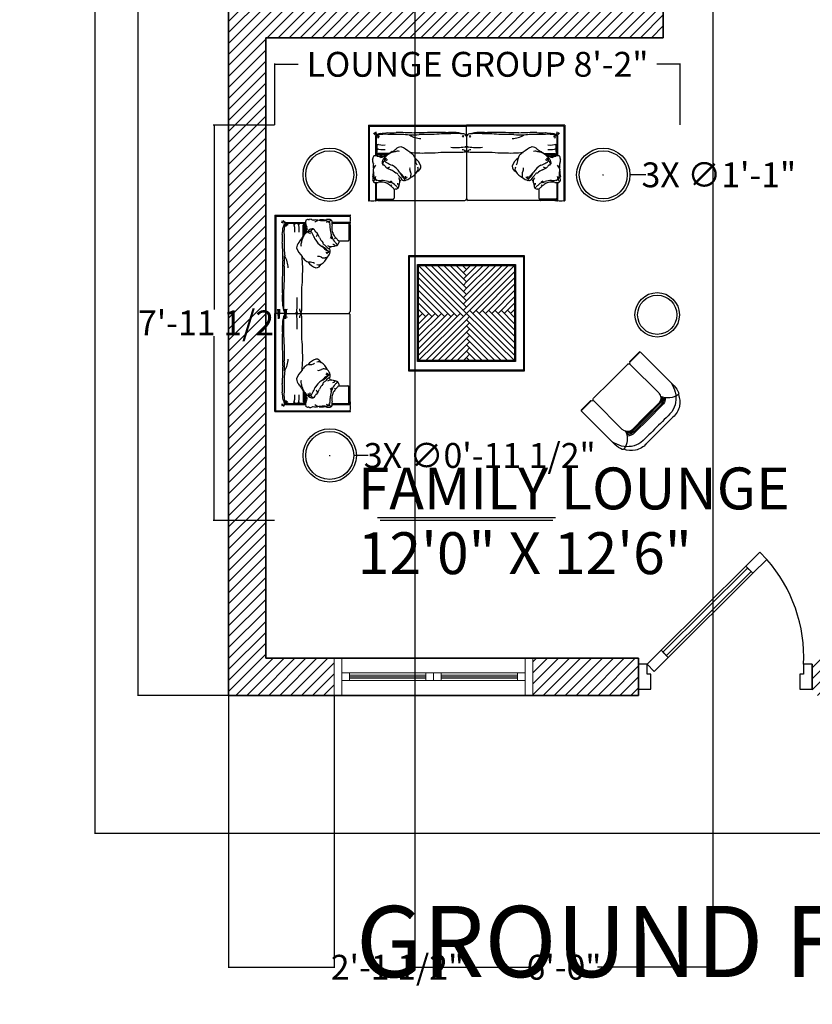
# Model space of a CAD drawing. Units: inches. Extents: x 585 to 1401, y -184 to 463.
# Tile 1 of 8: x 604 to 796, y -184 to 53. Entities that reach past the tile are written whole.
import ezdxf

# ---------------------------------------------------------------- set-up
doc = ezdxf.new("R2010")
doc.units = ezdxf.units.IN
doc.header["$MEASUREMENT"] = 0
for name, color, linetype, lineweight in [('A-ANNO-DIMS', 2, 'Continuous', 18), ('A-ANNO-TEXT', 7, 'Continuous', 25), ('A-AREA-IDEN', 7, 'Continuous', 18), ('A-Door', 150, 'Continuous', 25), ('A-FURN', 8, 'Continuous', 18), ('A-Glaz', 140, 'Continuous', 18), ('A-Wall', 7, 'Continuous', 35), ('A-WALL-PATT', 252, 'Continuous', 13)]:
    doc.layers.add(name, color=color, linetype=linetype, lineweight=lineweight)
doc.layers.add('furn', color=7, linetype='Continuous')
doc.styles.get("Standard").update_dxf_attribs({"font": 'arial.ttf'})
doc.dimstyles.get("Standard").update_dxf_attribs({"dimtxt": 6, "dimasz": 0.18, "dimexe": 0.18, "dimexo": 0.0625, "dimgap": 0.09, "dimtad": 0, "dimtih": 1, "dimtoh": 1, "dimdec": 0, "dimzin": 0, "dimdsep": 46, "dimlunit": 3, "dimtxsty": 'Standard', "dimblk": 'ARCHTICK', "dimcen": 0.09, "dimadec": 0, "dimazin": 0, "dimtfac": 1, "dimtdec": 0, "dimtofl": 0, "dimtmove": 0, "dimatfit": 3, "dimfxl": 1, "dimtolj": 1, "dimtzin": 0, "dimarcsym": 0})

# ---------------------------------------------------------------- blocks, each defined once
blk = doc.blocks.new('A$C1DF4181C')
blk.add_lwpolyline([(120, 128), (460.7, 466.1), (432.5, 494.5), (91.8, 156.4)], close=True)
blk.add_arc((72.4, 128.7), 593.3, 357.2313, 41.4937)
at = {"layer": 'A-Door'}
for points in [[(517.5, 522.4), (460.7, 466.1), (432.5, 494.5), (489.3, 550.8)], [(63.2, 71.6), (120, 128), (91.8, 156.4), (35, 100)], [(35, 100), (0, 100), (0, 0), (50, 0), (50, 50), (50, 60), (35, 60)], [(665, 100), (665, 60), (650, 60), (650, 50), (650, 0), (700, 0), (700, 100)]]:
    blk.add_lwpolyline(points, close=True, dxfattribs=at)
at = {"layer": 'A-Glaz'}
blk.add_lwpolyline([(112.9, 135.1), (453.6, 473.2), (439.5, 487.4), (98.8, 149.3)], close=True, dxfattribs=at)
at = {"layer": 'A-Wall'}
for p, q in [((0, 0), (0, 100)), ((0, 100), (0, 0)), ((700, 0), (700, 100)), ((700, 0), (700, 100))]:
    blk.add_line(p, q, dxfattribs=at)
blk = doc.blocks.new('CHAIR20')
at = {"layer": 'furn'}
for p, q in [((-0.211, 0.78), (0, 0.78)), ((0.211, 0.78), (0, 0.78)), ((-0.215, 0.6), (0, 0.6)), ((-0.215, 0.586), (0, 0.586)), ((-0.215, 0.57), (0, 0.57)), ((-0.215, 0.563), (0, 0.563)), ((-0.215, 0.556), (0, 0.556)), ((0.215, 0.6), (0, 0.6)), ((0.215, 0.586), (0, 0.586)), ((0.215, 0.57), (0, 0.57)), ((0.215, 0.563), (0, 0.563)), ((0.215, 0.556), (0, 0.556)), ((-0.47, 0), (-0.468, 0.541)), ((-0.29, 0.021), (-0.29, 0.475)), ((0.29, 0.021), (0.29, 0.475)), ((0.47, 0), (0.468, 0.541)), ((-0.469, 0), (-0.31, 0)), ((0, 0), (-0.27, 0)), ((0, 0), (0.27, 0)), ((0.469, 0), (0.31, 0)), ((-0.47, -0.005), (-0.31, -0.005)), ((0.47, -0.005), (0.31, -0.005))]:
    blk.add_line(p, q, dxfattribs=at)
for centre, radius, start, end in [((-0.231, 0.565), 0.216, 84.7548, 123.4097), ((0.231, 0.565), 0.216, 56.5903, 95.2452), ((-0.223, 0.553), 0.23, 123.4545, 156.6889), ((-0.195, 0.46), 0.272, 100.5852, 148.7439), ((-0.109, -1.87), 2.601, 87.5932, 92.9868), ((0.109, -1.87), 2.601, 87.0132, 92.4068), ((0.195, 0.46), 0.272, 31.2561, 79.4148), ((0.223, 0.553), 0.23, 23.3111, 56.5455), ((-0.233, 0.541), 0.236, 156.5177, 180), ((0.007, 0.371), 0.492, 152.1805, 165.4655), ((-0.419, 0.606), 0.0407, 111.0099, 136.0664), ((-0.467, 0.444), 0.203, 20.9169, 80.6589), ((-0.222, 0.487), 0.114, 86.6035, 136.5485), ((-0.216, 0.477), 0.109, 89.2329, 136.3875), ((-0.204, 0.471), 0.086, 97.254, 176.9258), ((-0.216, 0.47), 0.1, 89.4632, 135.7499), ((-0.21, 0.462), 0.101, 92.9164, 137.0487), ((0.223, 0.495), 0.106, 40.7338, 94.3098), ((0.217, 0.48), 0.106, 42.5807, 91.1067), ((0.22, 0.489), 0.0812, 35.3841, 93.3578), ((0.215, 0.483), 0.0803, 33.6859, 89.9707), ((0.204, 0.471), 0.086, 3.0742, 82.746), ((0.467, 0.444), 0.203, 99.3411, 159.0831), ((-0.007, 0.371), 0.492, 14.5345, 27.8195), ((0.419, 0.606), 0.0407, 43.9336, 68.9901), ((0.233, 0.541), 0.236, 360, 23.4823), ((-0.31, -0.003), 0.0025, 270, 90), ((-0.318, 0.028), 0.0294, 288.7273, 346.2133), ((-0.27, 0.02), 0.0204, 180, 270), ((0.27, 0.02), 0.0204, 270, 0), ((0.318, 0.028), 0.0294, 193.7867, 251.2727), ((0.31, -0.003), 0.0025, 90, 270)]:
    blk.add_arc(centre, radius, start, end, dxfattribs=at)
blk = doc.blocks.new('COUCH19')
at = {"layer": 'furn'}
for p, q in [((-1.104, 0), (0, 0)), ((-1.104, 0), (-1.104, -0.846)), ((1.104, 0), (0, 0)), ((1.104, 0), (1.104, -0.846)), ((-1.094, -0.01), (0, -0.01)), ((-1.094, -0.01), (-1.094, -0.846)), ((1.094, -0.01), (0, -0.01)), ((0, -0.129), (0, -0.01)), ((0, -0.129), (0, -0.01)), ((1.094, -0.01), (1.094, -0.846)), ((-1.023, -0.121), (-1.023, -0.343)), ((-1.015, -0.121), (-1.015, -0.343)), ((0, -0.129), (0, -0.827)), ((0, -0.129), (0, -0.827)), ((1.015, -0.121), (1.015, -0.343)), ((1.023, -0.121), (1.023, -0.343)), ((-0.881, -0.327), (-1.002, -0.327)), ((-0.872, -0.32), (-0.994, -0.32)), ((0.872, -0.32), (0.994, -0.32)), ((0.881, -0.327), (1.002, -0.327)), ((-0.891, -0.335), (-1.007, -0.335)), ((0.891, -0.335), (1.007, -0.335)), ((-1.039, -0.623), (-1.034, -0.607)), ((-1.034, -0.607), (-1.034, -0.6)), ((-1.025, -0.646), (-1.025, -0.846)), ((-1.015, -0.646), (-1.015, -0.821)), ((1.015, -0.646), (1.015, -0.821)), ((1.025, -0.646), (1.025, -0.846)), ((1.034, -0.607), (1.034, -0.6)), ((1.039, -0.623), (1.034, -0.607)), ((-0.814, -0.722), (-0.814, -0.821)), ((0.814, -0.722), (0.814, -0.821)), ((-1.015, -0.821), (-1.015, -0.846)), ((-0.995, -0.847), (-1.015, -0.846)), ((-1.005, -0.831), (-0.824, -0.831)), ((-1.005, -0.837), (-0.995, -0.837)), ((-0.995, -0.837), (-0.831, -0.837)), ((-0.995, -0.847), (-0.02, -0.847)), ((-0.824, -0.837), (-0.831, -0.837)), ((0.995, -0.847), (0.02, -0.847)), ((1.005, -0.831), (0.824, -0.831)), ((0.824, -0.837), (0.831, -0.837)), ((0.995, -0.837), (0.831, -0.837)), ((1.005, -0.837), (0.995, -0.837)), ((0.995, -0.847), (1.015, -0.846)), ((1.015, -0.821), (1.015, -0.846))]:
    blk.add_line(p, q, dxfattribs=at)
for centre, radius, start, end in [((-1.048, -0.115), 0.0203, 17.0736, 84.3161), ((-0.968, -0.057), 0.0723, 198.2313, 214.9565), ((-1.009, -0.12), 0.0145, 57.2943, 186.5462), ((-0.913, -0.069), 0.108, 182.4523, 195.8536), ((-0.96, -0.21), 0.104, 90.0493, 121.9997), ((-0.996, -0.106), 0.00486, 122.7707, 200.3161), ((-0.966, -0.156), 0.0629, 94.3136, 120.9365), ((-1.423, 4.307), 4.423, 275.8579, 276.9681), ((-0.915, -0.433), 0.331, 85.1525, 97.9068), ((-1.082, -27.361), 27.258, 89.2493, 89.5898), ((-0.842, 0.214), 0.301, 261.6444, 279.9904), ((-0.9, -7.819), 7.737, 87.6972, 89.1894), ((-0.72, -0.634), 0.528, 81.9914, 90.5051), ((-0.667, 1.941), 2.051, 270.5757, 273.7762), ((-0.512, 0.093), 0.242, 237.1993, 269.7033), ((-0.319, -8.828), 8.745, 89.7845, 91.769), ((-0.33, -15.825), 15.721, 90.2143, 90.7368), ((-0.087, -4.683), 4.588, 91.1175, 93.7755), ((-0.266, -0.71), 0.627, 85.799, 91.817), ((-0.14, -1.25), 1.168, 90.3024, 93.9345), ((-0.126, -1.263), 1.168, 85.3696, 92.4609), ((-0.166, -0.628), 0.546, 75.7588, 87.926), ((-0.04, -0.139), 0.0409, 14.1276, 78.4905), ((0.04, -0.139), 0.0409, 101.5095, 165.8724), ((0.166, -0.628), 0.546, 92.074, 104.2412), ((0.126, -1.263), 1.168, 87.5391, 94.6304), ((0.14, -1.25), 1.168, 86.0655, 89.6976), ((0.087, -4.683), 4.588, 86.2245, 88.8825), ((0.266, -0.71), 0.627, 88.183, 94.201), ((0.319, -8.828), 8.745, 88.231, 90.2155), ((0.33, -15.825), 15.721, 89.2632, 89.7857), ((0.512, 0.093), 0.242, 270.2967, 302.8007), ((0.667, 1.941), 2.051, 266.2238, 269.4243), ((0.9, -7.819), 7.737, 90.8106, 92.3028), ((0.72, -0.634), 0.528, 89.4949, 98.0086), ((1.082, -27.361), 27.258, 90.4102, 90.7507), ((0.842, 0.214), 0.301, 260.0096, 278.3556), ((1.423, 4.307), 4.423, 263.0319, 264.1421), ((0.915, -0.433), 0.331, 82.0932, 94.8475), ((0.96, -0.21), 0.104, 58.0003, 89.9507), ((0.966, -0.156), 0.0629, 59.0635, 85.6864), ((0.996, -0.106), 0.00486, 339.6839, 57.2293), ((1.009, -0.12), 0.0145, 353.4538, 122.7057), ((0.913, -0.069), 0.108, 344.1464, 357.5477), ((0.968, -0.057), 0.0723, 325.0435, 341.7687), ((1.048, -0.115), 0.0203, 95.6839, 162.9264), ((-0.939, 0.027), 0.251, 252.3074, 275.6547), ((-0.994, -0.25), 0.0327, 92.9653, 130.6064), ((-0.894, -0.245), 0.115, 167.1521, 190.1712), ((-0.964, -0.099), 0.0448, 212.1595, 236.9331), ((-0.856, -0.07), 0.158, 202.4283, 209.546), ((-0.97, -0.086), 0.0431, 234.5258, 258.9374), ((-0.073, -0.098), 0.0376, 311.3275, 340.0315), ((-0.008, -0.14), 0.0347, 134.9326, 177.5735), ((0.008, -0.14), 0.0347, 2.4265, 45.0674), ((0.073, -0.098), 0.0376, 199.9685, 228.6725), ((0.939, 0.027), 0.251, 264.3453, 287.6926), ((0.97, -0.086), 0.0431, 281.0626, 305.4742), ((0.964, -0.099), 0.0448, 303.0669, 327.8405), ((0.856, -0.07), 0.158, 330.454, 337.5717), ((0.994, -0.25), 0.0327, 49.3936, 87.0347), ((0.894, -0.245), 0.115, 349.8288, 12.8479), ((-0.939, -0.024), 0.251, 252.3074, 275.6547), ((-0.994, -0.301), 0.0327, 92.9653, 130.6064), ((-0.857, -0.308), 0.154, 166.0216, 193.8638), ((-0.973, -0.351), 0.0372, 124.129, 155.6456), ((-0.64, -0.622), 0.381, 121.3884, 141.1262), ((-0.778, -0.489), 0.191, 103.8154, 126.1732), ((-0.87, -0.199), 0.102, 288.1097, 316.2167), ((-0.809, -0.329), 0.0295, 76.0234, 121.4473), ((-0.771, -0.355), 0.0628, 74.6366, 119.4928), ((-0.724, -0.349), 0.107, 96.6363, 132.3883), ((-0.88, -0.576), 0.363, 48.2458, 66.6988), ((-0.503, 0.934), 1.247, 263.7654, 274.0351), ((-0.725, -0.457), 0.175, 42.4762, 60.188), ((-0.725, -0.457), 0.175, 42.4762, 60.188), ((-0.375, 0.101), 0.413, 264.3547, 281.9389), ((-0.196, 4.611), 4.915, 268.9098, 270.7856), ((-0.119, 0.604), 0.855, 266.0301, 276.6241), ((-0.098, 0.811), 1.115, 268.4407, 274.3812), ((-0.044, -0.31), 0.0328, 17.7761, 99.4289), ((-0.107, -0.054), 0.211, 294.188, 300.3458), ((-0.022, -0.281), 0.0348, 51.0228, 87.0896), ((-0.031, -0.275), 0.031, 305.699, 355.589), ((0.107, -0.054), 0.211, 239.6542, 245.812), ((0.022, -0.281), 0.0348, 92.9104, 128.9772), ((0.031, -0.275), 0.031, 184.411, 234.301), ((0.044, -0.31), 0.0328, 80.5711, 162.2239), ((0.098, 0.811), 1.115, 265.6188, 271.5593), ((0.119, 0.604), 0.855, 263.3759, 273.9699), ((0.196, 4.611), 4.915, 269.2144, 271.0902), ((0.375, 0.101), 0.413, 258.0611, 275.6453), ((0.503, 0.934), 1.247, 265.9649, 276.2346), ((0.725, -0.457), 0.175, 119.812, 137.5238), ((0.725, -0.457), 0.175, 119.812, 137.5238), ((0.88, -0.576), 0.363, 113.3012, 131.7542), ((0.724, -0.349), 0.107, 47.6117, 83.3637), ((0.771, -0.355), 0.0628, 60.5072, 105.3634), ((0.87, -0.199), 0.102, 223.7833, 251.8903), ((0.809, -0.329), 0.0295, 58.5527, 103.9766), ((0.778, -0.489), 0.191, 53.8268, 76.1846), ((0.64, -0.622), 0.381, 38.8738, 58.6116), ((0.939, -0.024), 0.251, 264.3453, 287.6926), ((0.973, -0.351), 0.0372, 24.3544, 55.871), ((0.994, -0.301), 0.0327, 49.3936, 87.0347), ((0.857, -0.308), 0.154, 346.1362, 13.9784), ((-1.074, -0.38), 0.0201, 328.1289, 14.357), ((-0.994, -0.395), 0.0636, 175.6653, 199.8843), ((-1.018, -0.373), 0.0366, 132.1042, 182.6049), ((-1.086, -0.435), 0.0374, 5.6263, 29.8671), ((-0.86, -0.46), 0.19, 171.4675, 186.7529), ((-1.02, -0.443), 0.0992, 87.1233, 102.9613), ((-1.013, -0.353), 0.00989, 37.5822, 102.987), ((-1.015, -0.343), 9e-16, 206.5651, 285.6691), ((-0.806, 2.328), 2.683, 265.7407, 267.224), ((-1.015, -0.433), 0.0861, 60.7186, 83.3154), ((-0.96, -0.34), 0.0224, 233.3829, 291.8634), ((-1.809, -0.344), 0.841, 359.8911, 0.568), ((-1.804, -0.344), 0.841, 359.8911, 0.568), ((-1.799, -0.344), 0.841, 359.8911, 0.568), ((-0.948, -0.373), 0.013, 53.2477, 107.2116), ((-0.93, -0.425), 0.0209, 167.8442, 221.0322), ((-0.878, -0.426), 0.0721, 143.309, 175.5501), ((-1.79, -0.344), 0.841, 359.8911, 0.568), ((-0.898, -0.443), 0.0477, 118.9683, 174.6945), ((-0.931, -0.431), 0.0166, 205.7118, 264.9652), ((-0.477, 1.196), 1.614, 253.4667, 254.2703), ((-0.852, -0.338), 0.079, 177.9406, 186.4844), ((-0.835, -0.393), 0.0868, 155.8952, 185.312), ((-0.881, -0.376), 0.048, 211.7673, 255.8825), ((-0.839, -0.338), 0.079, 177.9406, 186.4844), ((-0.89, -0.395), 0.0251, 116.2153, 179.4697), ((-0.831, -0.338), 0.079, 177.9406, 186.4844), ((-0.886, -0.413), 0.0239, 98.1103, 149.2033), ((-0.595, 0.089), 0.592, 239.8006, 245.8501), ((-0.668, -0.399), 0.0929, 9.1268, 39.8927), ((-0.683, -0.515), 0.178, 17.8257, 54.356), ((-0.465, -0.391), 0.111, 176.3175, 210.5975), ((0.683, -0.515), 0.178, 125.644, 162.1743), ((0.465, -0.391), 0.111, 329.4025, 3.6825), ((0.668, -0.399), 0.0929, 140.1073, 170.8732), ((0.595, 0.089), 0.592, 294.1499, 300.1994), ((0.886, -0.413), 0.0239, 30.7967, 81.8897), ((0.881, -0.376), 0.048, 284.1175, 328.2327), ((0.89, -0.395), 0.0251, 0.5303, 63.7847), ((0.831, -0.338), 0.079, 353.5156, 2.0594), ((0.477, 1.196), 1.614, 285.7297, 286.5333), ((0.835, -0.393), 0.0868, 354.688, 24.1048), ((0.839, -0.338), 0.079, 353.5156, 2.0594), ((0.898, -0.443), 0.0477, 5.3055, 61.0317), ((0.852, -0.338), 0.079, 353.5156, 2.0594), ((0.931, -0.431), 0.0166, 275.0348, 334.2882), ((0.806, 2.328), 2.683, 272.776, 274.2593), ((0.878, -0.426), 0.0721, 4.4499, 36.691), ((0.948, -0.373), 0.013, 72.7884, 126.7523), ((0.93, -0.425), 0.0209, 318.9678, 12.1558), ((1.79, -0.344), 0.841, 179.432, 180.1089), ((0.96, -0.34), 0.0224, 248.1366, 306.6171), ((1.799, -0.344), 0.841, 179.432, 180.1089), ((1.804, -0.344), 0.841, 179.432, 180.1089), ((1.809, -0.344), 0.841, 179.432, 180.1089), ((1.015, -0.433), 0.0861, 96.6846, 119.2814), ((1.013, -0.353), 0.00989, 77.013, 142.4178), ((1.02, -0.443), 0.0992, 77.0387, 92.8767), ((1.015, -0.343), 9e-16, 254.3309, 333.4349), ((1.018, -0.373), 0.0366, 357.3951, 47.8958), ((1.086, -0.435), 0.0374, 150.1329, 174.3737), ((0.86, -0.46), 0.19, 353.2471, 8.5325), ((0.994, -0.395), 0.0636, 340.1157, 4.3347), ((1.074, -0.38), 0.0201, 165.643, 211.8711), ((-1.182, -0.548), 0.131, 345.1133, 359.769), ((-0.686, -0.537), 0.366, 173.7033, 181.7891), ((-0.889, -0.546), 0.167, 144.4063, 162.8186), ((-0.984, -0.517), 0.0736, 131.9223, 151.7581), ((-1.323, -0.552), 0.28, 356.9803, 11.291), ((-0.95, -0.491), 0.0469, 30.0924, 67.7997), ((-0.868, -0.441), 0.0498, 212.7756, 251.3859), ((-0.896, -0.434), 0.0461, 267.613, 314.7931), ((-0.585, -0.588), 0.314, 159.3513, 161.4764), ((-0.167, 1.214), 1.847, 247.1663, 248.1939), ((-0.969, -0.731), 0.258, 48.2668, 63.2858), ((-0.962, -0.668), 0.251, 33.9468, 59.9573), ((-0.798, -0.569), 0.0309, 23.7706, 88.9158), ((-0.905, -0.702), 0.23, 28.4078, 49.069), ((-0.431, -0.357), 0.366, 207.8284, 218.7759), ((-0.564, -0.49), 0.0765, 172.087, 207.6691), ((-0.691, -0.443), 0.158, 291.3084, 330.3796), ((-0.669, -0.55), 0.0453, 340.7695, 33.0701), ((-0.578, -0.461), 0.0648, 291.8488, 0.3181), ((-0.593, -0.493), 0.0481, 323.948, 24.7103), ((0.578, -0.461), 0.0648, 179.6819, 248.1512), ((0.593, -0.493), 0.0481, 155.2897, 216.052), ((0.691, -0.443), 0.158, 209.6204, 248.6916), ((0.669, -0.55), 0.0453, 146.9299, 199.2305), ((0.564, -0.49), 0.0765, 332.3309, 7.913), ((0.905, -0.702), 0.23, 130.931, 151.5922), ((0.431, -0.357), 0.366, 321.2241, 332.1716), ((0.962, -0.668), 0.251, 120.0427, 146.0532), ((0.798, -0.569), 0.0309, 91.0842, 156.2294), ((0.969, -0.731), 0.258, 116.7142, 131.7332), ((0.167, 1.214), 1.847, 291.8061, 292.8337), ((0.896, -0.434), 0.0461, 225.2069, 272.387), ((0.585, -0.588), 0.314, 18.5236, 20.6487), ((0.868, -0.441), 0.0498, 288.6141, 327.2244), ((0.95, -0.491), 0.0469, 112.2003, 149.9076), ((0.889, -0.546), 0.167, 17.1814, 35.5937), ((0.984, -0.517), 0.0736, 28.2419, 48.0777), ((1.323, -0.552), 0.28, 168.709, 183.0197), ((0.686, -0.537), 0.366, 358.2109, 6.2967), ((1.182, -0.548), 0.131, 180.231, 194.8867), ((-1.024, -0.613), 0.0321, 161.9809, 225.4662), ((-0.893, -0.587), 0.162, 178.3049, 185.9426), ((-1.03, -0.629), 0.0178, 205.5377, 287.1664), ((-0.992, -0.65), 0.0551, 132.3214, 167.2209), ((-0.897, -0.539), 0.15, 190.4981, 208.008), ((-0.912, -0.624), 0.12, 156.9441, 171.4926), ((-1.03, -0.627), 0.021, 40.1938, 92.7238), ((-1.008, -0.595), 0.0252, 215.3505, 284.8971), ((-1.02, -0.49), 0.156, 268.1697, 279.3739), ((-0.956, -0.246), 0.376, 262.9976, 269.9218), ((-0.962, -0.86), 0.219, 83.6792, 98.7215), ((-0.944, -0.776), 0.154, 66.7964, 94.5064), ((-0.932, -0.683), 0.0412, 54.7023, 97.6283), ((-0.917, -0.717), 0.0675, 38.8585, 82.2417), ((-0.872, -0.602), 0.0345, 250.3736, 320.202), ((-0.845, -0.558), 0.0857, 243.3753, 262.8098), ((-0.856, -0.621), 0.0218, 270.7288, 323.4039), ((-0.889, -0.757), 0.119, 41.7125, 74.0479), ((-0.746, -0.653), 0.0296, 176.2272, 243.906), ((-0.704, -0.523), 0.0736, 207.4289, 240.3049), ((-1.045, -0.616), 0.293, 343.2655, 351.5283), ((-0.824, -0.632), 0.074, 338.2529, 34.2498), ((-0.708, -0.654), 0.0475, 113.0369, 152.7943), ((-1.164, -0.867), 0.508, 30.4515, 33.5103), ((-0.703, -0.598), 0.0259, 206.1911, 303.1573), ((-0.725, -0.61), 0.0249, 24.0334, 69.6184), ((-0.757, -0.636), 0.07, 13.5386, 38.9825), ((-0.812, -0.683), 0.138, 27.1731, 37.2618), ((-0.707, -0.521), 0.101, 280.2692, 316.4215), ((-0.737, -0.592), 0.0518, 347.5061, 20.3402), ((-0.404, -0.825), 0.359, 137.003, 141.7232), ((-0.657, -0.57), 0.0307, 318.4165, 9.5076), ((0.657, -0.57), 0.0307, 170.4924, 221.5835), ((0.707, -0.521), 0.101, 223.5785, 259.7308), ((0.404, -0.825), 0.359, 38.2768, 42.997), ((0.737, -0.592), 0.0518, 159.6598, 192.4939), ((0.757, -0.636), 0.07, 141.0175, 166.4614), ((0.812, -0.683), 0.138, 142.7382, 152.8269), ((0.703, -0.598), 0.0259, 236.8427, 333.8089), ((0.725, -0.61), 0.0249, 110.3816, 155.9666), ((1.164, -0.867), 0.508, 146.4897, 149.5485), ((0.708, -0.654), 0.0475, 27.2057, 66.9631), ((0.704, -0.523), 0.0736, 299.6951, 332.5711), ((0.824, -0.632), 0.074, 145.7502, 201.7471), ((1.045, -0.616), 0.293, 188.4717, 196.7345), ((0.746, -0.653), 0.0296, 296.094, 3.7728), ((0.889, -0.757), 0.119, 105.9521, 138.2875), ((0.856, -0.621), 0.0218, 216.5961, 269.2712), ((0.872, -0.602), 0.0345, 219.798, 289.6264), ((0.845, -0.558), 0.0857, 277.1902, 296.6247), ((0.917, -0.717), 0.0675, 97.7583, 141.1415), ((0.944, -0.776), 0.154, 85.4936, 113.2036), ((0.932, -0.683), 0.0412, 82.3717, 125.2977), ((0.962, -0.86), 0.219, 81.2785, 96.3208), ((0.956, -0.246), 0.376, 270.0782, 277.0024), ((1.02, -0.49), 0.156, 260.6261, 271.8303), ((1.008, -0.595), 0.0252, 255.1029, 324.6495), ((1.03, -0.627), 0.021, 87.2762, 139.8062), ((0.912, -0.624), 0.12, 8.5074, 23.0559), ((1.03, -0.629), 0.0178, 252.8336, 334.4623), ((0.897, -0.539), 0.15, 331.992, 349.5019), ((0.992, -0.65), 0.0551, 12.7791, 47.6786), ((1.024, -0.613), 0.0321, 314.5338, 18.0191), ((0.893, -0.587), 0.162, 354.0574, 1.6951), ((-0.941, -0.799), 0.146, 43.1034, 58.5529), ((-0.853, -0.666), 0.0145, 257.1917, 333.3739), ((-0.893, -0.772), 0.0937, 32.4441, 51.2679), ((-0.8, -0.74), 0.0226, 72.9422, 128.2888), ((-0.836, -0.734), 0.0664, 30.0116, 56.9073), ((-0.799, -0.676), 0.0425, 277.944, 324.851), ((-0.776, -0.683), 0.0176, 263.1309, 322.8554), ((0.776, -0.683), 0.0176, 217.1446, 276.8691), ((0.799, -0.676), 0.0425, 215.149, 262.056), ((0.836, -0.734), 0.0664, 123.0927, 149.9884), ((0.8, -0.74), 0.0226, 51.7112, 107.0578), ((0.893, -0.772), 0.0937, 128.7321, 147.5559), ((0.941, -0.799), 0.146, 121.4471, 136.8966), ((0.853, -0.666), 0.0145, 206.6261, 282.8083), ((-1.099, -0.846), 0.00498, 180, 0), ((-1.059, -0.763), 0.0891, 247.4155, 292.5845), ((-1.02, -0.846), 0.00498, 180, 0), ((-1.005, -0.821), 0.00996, 180, 270), ((-1.005, -0.834), 0.00308, 90, 270), ((-0.995, -0.842), 0.00481, 90, 270), ((-0.831, -0.842), 0.00481, 270, 90), ((-0.824, -0.821), 0.00996, 270, 360), ((-0.824, -0.834), 0.00308, 270, 90), ((-0.02, -0.827), 0.0199, 270, 360), ((0.02, -0.827), 0.0199, 180, 270), ((0.824, -0.821), 0.00996, 180, 270), ((0.824, -0.834), 0.00308, 90, 270), ((0.831, -0.842), 0.00481, 90, 270), ((0.995, -0.842), 0.00481, 270, 90), ((1.005, -0.821), 0.00996, 270, 0), ((1.005, -0.834), 0.00308, 270, 90), ((1.02, -0.846), 0.00498, 180, 0), ((1.059, -0.763), 0.0891, 247.4155, 292.5845), ((1.099, -0.846), 0.00498, 180, 0)]:
    blk.add_arc(centre, radius, start, end, dxfattribs=at)
blk = doc.blocks.new('TABLE24')
at = {"layer": 'furn'}
for p, q in [((0, -1.3), (0, 0)), ((0, 0), (1.3, 0)), ((1.3, 0), (1.3, -1.3)), ((0.01, -1.29), (0.01, -0.01)), ((0.01, -0.01), (1.29, -0.01)), ((0.1, -1.2), (0.1, -0.1)), ((0.1, -0.1), (1.19, -0.1)), ((0.11, -1.19), (0.11, -0.11)), ((0.11, -0.11), (1.18, -0.11)), ((0.65, -0.65), (0.11, -0.11)), ((0.65, -0.579), (0.181, -0.11)), ((0.65, -0.509), (0.251, -0.11)), ((0.65, -0.438), (0.322, -0.11)), ((0.65, -0.367), (0.393, -0.11)), ((0.65, -0.296), (0.464, -0.11)), ((0.65, -0.226), (0.534, -0.11)), ((0.65, -0.155), (0.605, -0.11)), ((1.119, -0.11), (0.615, -0.615)), ((1.049, -0.11), (0.615, -0.544)), ((0.978, -0.11), (0.615, -0.473)), ((0.907, -0.11), (0.615, -0.403)), ((0.836, -0.11), (0.615, -0.332)), ((0.766, -0.11), (0.615, -0.261)), ((0.695, -0.11), (0.615, -0.19)), ((0.624, -0.11), (0.615, -0.12)), ((1.18, -0.11), (0.65, -0.65)), ((1.18, -0.11), (1.18, -1.19)), ((1.19, -0.1), (1.19, -1.2)), ((1.29, -0.01), (1.29, -1.29)), ((0.579, -0.65), (0.11, -0.181)), ((1.18, -0.191), (0.721, -0.65)), ((0.509, -0.65), (0.11, -0.251)), ((0.438, -0.65), (0.11, -0.322)), ((1.18, -0.261), (0.791, -0.65)), ((0.367, -0.65), (0.11, -0.393)), ((1.18, -0.332), (0.862, -0.65)), ((1.18, -0.403), (0.933, -0.65)), ((0.296, -0.65), (0.11, -0.464)), ((0.261, -0.685), (0.11, -0.534)), ((1.18, -0.474), (1.004, -0.65)), ((1.18, -0.544), (1.074, -0.65)), ((0.19, -0.685), (0.11, -0.605)), ((0.65, -0.65), (0.11, -1.19)), ((0.509, -0.65), (0.11, -1.049)), ((0.579, -0.65), (0.11, -1.119)), ((0.438, -0.65), (0.11, -0.978)), ((0.296, -0.65), (0.11, -0.836)), ((0.367, -0.65), (0.11, -0.907)), ((0.226, -0.65), (0.11, -0.766)), ((0.155, -0.65), (0.11, -0.695)), ((0.332, -0.685), (0.296, -0.65)), ((0.403, -0.685), (0.367, -0.65)), ((0.473, -0.685), (0.438, -0.65)), ((0.544, -0.685), (0.509, -0.65)), ((0.615, -0.685), (0.579, -0.65)), ((1.18, -1.19), (0.65, -0.65)), ((0.721, -0.65), (0.685, -0.615)), ((1.18, -1.109), (0.721, -0.65)), ((0.791, -0.65), (0.756, -0.615)), ((1.18, -1.039), (0.791, -0.65)), ((0.862, -0.65), (0.827, -0.615)), ((1.18, -0.968), (0.862, -0.65)), ((0.933, -0.65), (0.897, -0.615)), ((1.18, -0.897), (0.933, -0.65)), ((1.004, -0.65), (0.968, -0.615)), ((1.18, -0.826), (1.004, -0.65)), ((1.074, -0.65), (1.039, -0.615)), ((1.18, -0.756), (1.074, -0.65)), ((1.145, -0.65), (1.11, -0.615)), ((1.18, -0.615), (1.145, -0.65)), ((1.18, -0.685), (1.145, -0.65)), ((0.12, -0.685), (0.11, -0.676)), ((0.685, -0.685), (0.181, -1.19)), ((0.685, -0.756), (0.251, -1.19)), ((1.119, -1.19), (0.65, -0.721)), ((0.685, -0.827), (0.322, -1.19)), ((1.049, -1.19), (0.65, -0.791)), ((0.978, -1.19), (0.65, -0.862)), ((0.685, -0.897), (0.393, -1.19)), ((0.685, -0.968), (0.464, -1.19)), ((0.907, -1.19), (0.65, -0.933)), ((0.685, -1.039), (0.534, -1.19)), ((0.836, -1.19), (0.65, -1.004)), ((0.766, -1.19), (0.65, -1.074)), ((1.19, -1.2), (0.1, -1.2)), ((1.18, -1.19), (0.11, -1.19)), ((0.685, -1.11), (0.605, -1.19)), ((0.695, -1.19), (0.65, -1.145)), ((0.685, -1.18), (0.676, -1.19)), ((1.3, -1.3), (0, -1.3)), ((1.29, -1.29), (0.01, -1.29))]:
    blk.add_line(p, q, dxfattribs=at)
blk = doc.blocks.new('A$C42C86705')
at = {"layer": 'furn'}
for p, q in [((3.156, 0.03), (1.156, 0.03)), ((3.126, 0), (1.186, 0))]:
    blk.add_line(p, q, dxfattribs=at)
for centre, radius in [((0.617, 3.888), 0.3), ((0.617, 3.888), 0.27), ((3.694, 3.888), 0.3), ((3.694, 3.888), 0.27), ((4.301, 2.314), 0.25), ((4.301, 2.314), 0.22), ((0.617, 0.733), 0.3), ((0.617, 0.733), 0.27)]:
    blk.add_circle(centre, radius, dxfattribs=at)
blk.add_blockref('COUCH19', (2.156, 4.446), dxfattribs=at)
for name, p, rotation in [('COUCH19', (0, 2.33), 89.99999999999999), ('TABLE24', (2.806, 2.98), 270)]:
    blk.add_blockref(name, p, dxfattribs=dict(at, rotation=rotation))
at = {"layer": 'furn', "xscale": -1, "rotation": 225}
blk.add_blockref('CHAIR20', (3.777, 1.566), dxfattribs=at)
blk = doc.blocks.new('_ArchTick')
at = {"color": 0, "linetype": 'ByBlock', "const_width": 0.15}
blk.add_lwpolyline([(-0.5, -0.5), (0.5, 0.5)], dxfattribs=at)
blk = doc.blocks.new('*D27')
at = {"layer": 'A-ANNO-DIMS', "color": 0, "lineweight": -2, "transparency": 16777216}
for p, q in [((654.47, 422.15), (632.54, 422.15)), ((632.72, 422.15), (632.72, 159.24)), ((632.72, -109.85), (632.72, 153.06)), ((654.47, -109.85), (632.54, -109.85))]:
    blk.add_line(p, q, dxfattribs=at)
at = {"layer": 'Defpoints', "color": 0, "transparency": 16777216}
for p in [(654.53, 422.15), (632.72, -109.85), (654.53, -109.85)]:
    blk.add_point(p, dxfattribs=at)
at = {"layer": 'A-ANNO-DIMS', "color": 0, "lineweight": -2, "transparency": 16777216, "xscale": 0.18, "yscale": 0.18, "zscale": 0.18}
for p, rotation in [((632.72, 422.15), 90), ((632.72, -109.85), 270)]:
    blk.add_blockref('_ArchTick', p, dxfattribs=dict(at, rotation=rotation))
at = {"layer": 'A-ANNO-DIMS', "color": 0, "transparency": 16777216, "insert": (632.72, 156.15), "char_height": 6, "attachment_point": 5}
blk.add_mtext('\\A1;44\'-4"', dxfattribs=at)
blk = doc.blocks.new('WIN-48-DOUBLE-PANEL')
for p, q in [((48, 9), (0, 9)), ((0, 9), (0, 0)), ((1.85, 9), (0, 9)), ((0, 9), (0, 0)), ((1.85, 0), (1.85, 9)), ((1.85, 0), (1.85, 9)), ((46.15, 9), (48, 9)), ((46.15, 0), (46.15, 9)), ((46.15, 0), (46.15, 9)), ((46.15, 0), (46.15, 9)), ((48, 9), (48, 0)), ((48, 0), (48, 9)), ((1.85, 5.44), (46.15, 5.44)), ((3.69, 3.6), (3.69, 5.44)), ((3.69, 4.89), (22.15, 4.89)), ((22.15, 5.44), (22.15, 3.6)), ((24, 5.44), (24, 3.6)), ((25.85, 5.44), (25.85, 3.6)), ((44.31, 4.89), (25.85, 4.89)), ((44.31, 3.6), (44.31, 5.44)), ((1.85, 3.6), (46.15, 3.6)), ((3.69, 4.52), (22.15, 4.52)), ((3.69, 4.15), (22.15, 4.15)), ((44.31, 4.52), (25.85, 4.52)), ((44.31, 4.15), (25.85, 4.15)), ((0, 0), (1.85, 0)), ((48, 0), (0, 0)), ((48, 0), (46.15, 0))]:
    blk.add_line(p, q)
blk = doc.blocks.new('*D70')
at = {"layer": 'A-ANNO-DIMS', "color": 0, "lineweight": -2, "transparency": 16777216}
for p, q in [((665.71, 27.87), (665.71, 42.68)), ((665.71, 42.5), (671.34, 42.5)), ((763.62, 42.5), (757.99, 42.5)), ((763.62, 27.87), (763.62, 42.68))]:
    blk.add_line(p, q, dxfattribs=at)
at = {"layer": 'Defpoints', "color": 0, "transparency": 16777216}
for p in [(763.62, 42.5), (665.71, 27.81), (763.62, 27.81)]:
    blk.add_point(p, dxfattribs=at)
at = {"layer": 'A-ANNO-DIMS', "color": 0, "lineweight": -2, "transparency": 16777216, "xscale": 0.18, "yscale": 0.18, "zscale": 0.18, "rotation": 180}
blk.add_blockref('_ArchTick', (665.71, 42.5), dxfattribs=at)
at = {"layer": 'A-ANNO-DIMS', "color": 0, "lineweight": -2, "transparency": 16777216, "xscale": 0.18, "yscale": 0.18, "zscale": 0.18}
blk.add_blockref('_ArchTick', (763.62, 42.5), dxfattribs=at)
at = {"layer": 'A-ANNO-DIMS', "color": 0, "transparency": 16777216, "insert": (714.67, 42.5), "char_height": 6, "attachment_point": 5}
blk.add_mtext('\\A1;LOUNGE GROUP 8\'-2"', dxfattribs=at)
blk = doc.blocks.new('*D71')
at = {"layer": 'A-ANNO-DIMS', "color": 0, "lineweight": -2, "transparency": 16777216}
for p, q in [((665.65, 27.81), (650.84, 27.81)), ((651.02, 27.81), (651.02, -16.73)), ((651.02, -67.66), (651.02, -23.12)), ((665.65, -67.66), (650.84, -67.66))]:
    blk.add_line(p, q, dxfattribs=at)
at = {"layer": 'Defpoints', "color": 0, "transparency": 16777216}
for p in [(651.02, 27.81), (665.71, 27.81), (665.71, -67.66)]:
    blk.add_point(p, dxfattribs=at)
at = {"layer": 'A-ANNO-DIMS', "color": 0, "lineweight": -2, "transparency": 16777216, "xscale": 0.18, "yscale": 0.18, "zscale": 0.18}
for p, rotation in [((651.02, 27.81), 90), ((651.02, -67.66), 270)]:
    blk.add_blockref('_ArchTick', p, dxfattribs=dict(at, rotation=rotation))
at = {"layer": 'A-ANNO-DIMS', "color": 0, "transparency": 16777216, "insert": (651.02, -19.92), "char_height": 6, "attachment_point": 5}
blk.add_mtext('\\A1;7\'-11 1/2"', dxfattribs=at)
blk = doc.blocks.new('*D76')
at = {"layer": 'A-ANNO-DIMS', "color": 0, "lineweight": -2, "transparency": 16777216}
for p, q in [((654.47, 422.15), (622.1, 422.15)), ((622.28, 422.15), (622.28, 142.65)), ((622.28, -143.23), (622.28, 136.27)), ((807.47, -143.23), (622.1, -143.23))]:
    blk.add_line(p, q, dxfattribs=at)
at = {"layer": 'Defpoints', "color": 0, "transparency": 16777216}
for p in [(622.28, 422.15), (654.53, 422.15), (807.53, -143.23)]:
    blk.add_point(p, dxfattribs=at)
at = {"layer": 'A-ANNO-DIMS', "color": 0, "lineweight": -2, "transparency": 16777216, "xscale": 0.18, "yscale": 0.18, "zscale": 0.18}
for p, rotation in [((622.28, 422.15), 90), ((622.28, -143.23), 270)]:
    blk.add_blockref('_ArchTick', p, dxfattribs=dict(at, rotation=rotation))
at = {"layer": 'A-ANNO-DIMS', "color": 0, "transparency": 16777216, "insert": (622.28, 139.46), "char_height": 6, "attachment_point": 5}
blk.add_mtext('\\A1;47\'-1 1/2"', dxfattribs=at)
blk = doc.blocks.new('*D81')
at = {"layer": 'A-ANNO-DIMS', "color": 0, "lineweight": -2, "transparency": 16777216}
for p, q in [((699.53, 228.09), (699.53, -175.66)), ((771.53, 228.09), (771.53, -175.66)), ((699.53, -175.48), (727.45, -175.48)), ((771.53, -175.48), (743.61, -175.48))]:
    blk.add_line(p, q, dxfattribs=at)
at = {"layer": 'Defpoints', "color": 0, "transparency": 16777216}
for p in [(699.53, 228.15), (771.53, 228.15), (771.53, -175.48)]:
    blk.add_point(p, dxfattribs=at)
at = {"layer": 'A-ANNO-DIMS', "color": 0, "lineweight": -2, "transparency": 16777216, "xscale": 0.18, "yscale": 0.18, "zscale": 0.18, "rotation": 180}
blk.add_blockref('_ArchTick', (699.53, -175.48), dxfattribs=at)
at = {"layer": 'A-ANNO-DIMS', "color": 0, "lineweight": -2, "transparency": 16777216, "xscale": 0.18, "yscale": 0.18, "zscale": 0.18}
blk.add_blockref('_ArchTick', (771.53, -175.48), dxfattribs=at)
at = {"layer": 'A-ANNO-DIMS', "color": 0, "transparency": 16777216, "insert": (735.53, -175.48), "char_height": 6, "attachment_point": 5}
blk.add_mtext('\\A1;6\'-0"', dxfattribs=at)
blk = doc.blocks.new('*D87')
at = {"layer": 'A-ANNO-DIMS', "color": 0, "lineweight": -2, "transparency": 16777216}
for p, q in [((654.53, -109.91), (654.53, -175.66)), ((680.03, -109.91), (680.03, -175.66)), ((654.53, -175.48), (680.03, -175.48)), ((680.03, -175.48), (680.21, -175.48))]:
    blk.add_line(p, q, dxfattribs=at)
at = {"layer": 'Defpoints', "color": 0, "transparency": 16777216}
for p in [(654.53, -109.85), (680.03, -109.85), (680.03, -175.48)]:
    blk.add_point(p, dxfattribs=at)
at = {"layer": 'A-ANNO-DIMS', "color": 0, "lineweight": -2, "transparency": 16777216, "xscale": 0.18, "yscale": 0.18, "zscale": 0.18, "rotation": 180}
blk.add_blockref('_ArchTick', (654.53, -175.48), dxfattribs=at)
at = {"layer": 'A-ANNO-DIMS', "color": 0, "lineweight": -2, "transparency": 16777216, "xscale": 0.18, "yscale": 0.18, "zscale": 0.18}
blk.add_blockref('_ArchTick', (680.03, -175.48), dxfattribs=at)
at = {"layer": 'A-ANNO-DIMS', "color": 0, "transparency": 16777216, "insert": (695.31, -175.48), "char_height": 6, "attachment_point": 5}
blk.add_mtext('\\A1;2\'-1 1/2"', dxfattribs=at)
blk = doc.blocks.new('*D99')
at = {"layer": 'A-ANNO-DIMS', "color": 0, "lineweight": -2, "transparency": 16777216}
for p, q in [((744.93, 15.82), (745.11, 15.82)), ((745.02, 15.73), (745.02, 15.91)), ((755.33, 15.82), (751.46, 15.82))]:
    blk.add_line(p, q, dxfattribs=at)
at = {"layer": 'Defpoints', "color": 0, "transparency": 16777216}
for p in [(738.58, 15.82), (751.46, 15.82)]:
    blk.add_point(p, dxfattribs=at)
at = {"layer": 'A-ANNO-DIMS', "color": 0, "lineweight": -2, "transparency": 16777216, "xscale": 0.18, "yscale": 0.18, "zscale": 0.18, "rotation": 179.998630246816}
blk.add_blockref('_ArchTick', (751.46, 15.82), dxfattribs=at)
at = {"layer": 'A-ANNO-DIMS', "color": 0, "transparency": 16777216, "insert": (772.94, 15.82), "char_height": 6, "attachment_point": 5}
blk.add_mtext('\\A1;3X ∅1\'-1"', dxfattribs=at)
blk = doc.blocks.new('*D100')
at = {"layer": 'A-ANNO-DIMS', "color": 0, "lineweight": -2, "transparency": 16777216}
for p, q in [((678.88, -51.93), (679.06, -51.93)), ((678.97, -52.02), (678.97, -51.84)), ((688.24, -51.93), (684.77, -51.93))]:
    blk.add_line(p, q, dxfattribs=at)
at = {"layer": 'Defpoints', "color": 0, "transparency": 16777216}
for p in [(673.17, -51.93), (684.77, -51.93)]:
    blk.add_point(p, dxfattribs=at)
at = {"layer": 'A-ANNO-DIMS', "color": 0, "lineweight": -2, "transparency": 16777216, "xscale": 0.18, "yscale": 0.18, "zscale": 0.18, "rotation": 179.9979443818756}
blk.add_blockref('_ArchTick', (684.77, -51.93), dxfattribs=at)
at = {"layer": 'A-ANNO-DIMS', "color": 0, "transparency": 16777216, "insert": (715.18, -51.93), "char_height": 6, "attachment_point": 5}
blk.add_mtext('\\A1;3X ∅0\'-11 1/2"', dxfattribs=at)

msp = doc.modelspace()

# ---------------------------------------------------------------- hatches: boundary and pattern name
at = {"layer": 'A-WALL-PATT'}
h = msp.add_hatch(dxfattribs=at)
h.set_pattern_fill('ANSI31', color=256, scale=15)
h.set_pattern_definition([(45, (599.059, -1e-14), (-1.325825, 1.325825), [])])
h.paths.add_polyline_path([(711.53, 422.15), (654.53, 422.15), (654.53, -109.85), (680.03, -109.85), (680.03, -100.85), (663.53, -100.85), (663.53, 48.87), (759.53, 48.87), (759.53, 57.87), (663.53, 57.87), (663.53, 144.15), (663.53, 264.15), (812.53, 264.15), (812.53, 269.15), (663.53, 269.15), (663.53, 413.15), (711.53, 413.15)])
h.paths.add_polyline_path([(753.53, -100.85), (728.03, -100.85), (728.03, -109.85), (753.53, -109.85)], flags=17)
h.paths.add_polyline_path([(812.53, -71.54), (807.53, -71.54), (807.53, -100.85), (795.53, -100.85), (795.53, -109.85), (807.53, -109.85), (807.53, -143.23), (848.53, -143.23), (848.53, -134.23), (812.53, -134.23)])
h.paths.add_polyline_path([(941.53, 8.77), (932.53, 8.77), (932.53, -9.23), (812.53, -9.23), (812.53, 5.77), (807.53, 5.77), (807.53, -29.54), (812.53, -29.54), (812.53, -14.23), (932.53, -14.23), (932.53, -134.23), (896.53, -134.23), (896.53, -143.23), (941.53, -143.23)])
h.paths.add_polyline_path([(941.53, 91.77), (932.53, 91.77), (932.53, 55.77), (812.53, 55.77), (812.53, 98.58), (807.53, 98.58), (807.53, 35.77), (812.53, 35.77), (812.53, 50.77), (932.53, 50.77), (932.53, 32.77), (941.53, 32.77)])
h.paths.add_polyline_path([(941.53, 222.04), (932.53, 222.04), (932.53, 180.77), (807.53, 180.77), (807.53, 140.58), (812.53, 140.58), (812.53, 175.77), (932.53, 175.77), (932.53, 139.77), (941.53, 139.77)])
h.paths.add_polyline_path([(941.53, 422.15), (896.53, 422.15), (896.53, 413.15), (932.53, 413.15), (932.53, 317.15), (896.53, 317.15), (896.53, 312.15), (932.53, 312.15), (932.53, 270.04), (941.53, 270.04)])
h.paths.add_polyline_path([(848.53, 422.15), (759.53, 422.15), (759.53, 413.15), (807.53, 413.15), (807.53, 312.15), (848.53, 312.15), (848.53, 317.15), (812.53, 317.15), (812.53, 413.15), (848.53, 413.15)])

# ---------------------------------------------------------------- linework, layer by layer
at = {"layer": 'A-Wall'}
for p, q in [((654.53, 422.15), (654.53, -109.85)), ((759.53, 57.87), (759.53, 48.87)), ((759.53, 48.87), (663.53, 48.87)), ((663.53, 48.87), (663.53, -100.85)), ((663.53, -100.85), (753.53, -100.85)), ((753.53, -100.85), (753.53, -109.85)), ((654.53, -109.85), (753.53, -109.85))]:
    msp.add_line(p, q, dxfattribs=at)

# ---------------------------------------------------------------- block references
at = {"layer": 'A-Door', "xscale": 0.0599999999683043, "yscale": 0.0599999999683043, "zscale": 0.0599999999683043}
msp.add_blockref('A$C1DF4181C', (753.53, -108.35), dxfattribs=at)
at = {"layer": 'A-FURN', "xscale": 21.4723583840094, "yscale": 21.4723583840094, "zscale": 21.4723583840094}
msp.add_blockref('A$C42C86705', (665.71, -67.66), dxfattribs=at)
at = {"layer": 'A-Glaz'}
msp.add_blockref('WIN-48-DOUBLE-PANEL', (680.03, -109.85), dxfattribs=at)

# ---------------------------------------------------------------- texts
at = {"layer": 'A-ANNO-TEXT'}
msp.add_text('GROUND FLOOR', height=17.1732, dxfattribs=at).set_placement((685.33, -177.86))
at = {"layer": 'A-AREA-IDEN'}
for s, p in [('FAMILY LOUNGE', (685.73, -64.94)), ('12\'0" X 12\'6"', (685.73, -80.57))]:
    msp.add_text(s, height=10.1013, dxfattribs=at).set_placement(p)

# ---------------------------------------------------------------- dimensions: what is measured, and where the dimension line sits
at = {"layer": 'A-ANNO-DIMS'}
for base, p1, p2, override, picture, middle in [((622.28, 422.15), (807.53, -143.23), (654.53, 422.15), {"dimdec": 1, "dimlfac": 1, "dimrnd": 0, "dimzin": 1, "dimdsep": 46, "dimlunit": 4, "dimfrac": 2}, '*D76', (622.28, 139.46)), ((632.72, -109.85), (654.53, 422.15), (654.53, -109.85), {"dimclrd": 0, "dimclre": 0, "dimclrt": 0}, '*D27', (632.72, 156.15)), ((651.02, 27.81), (665.71, -67.66), (665.71, 27.81), {"dimdec": 1, "dimlfac": 1, "dimrnd": 0, "dimzin": 1, "dimdsep": 46, "dimlunit": 4, "dimfrac": 2}, '*D71', (651.02, -19.92))]:
    dim = msp.add_linear_dim(base=base, p1=p1, p2=p2, angle=90, dimstyle='Standard', override=override, dxfattribs=at)
    dim.commit()
    dim.dimension.update_dxf_attribs({"geometry": picture, "text_midpoint": middle})
for base, p1, p2, picture, middle in [((771.53, -175.48), (699.53, 228.15), (771.53, 228.15), '*D81', (735.53, -175.48)), ((680.03, -175.48), (654.53, -109.85), (680.03, -109.85), '*D87', (695.31, -175.48))]:
    dim = msp.add_linear_dim(base=base, p1=p1, p2=p2, dimstyle='Standard', override={"dimdec": 1, "dimlfac": 1, "dimrnd": 0, "dimzin": 1, "dimdsep": 46, "dimlunit": 4, "dimfrac": 2}, dxfattribs=at)
    dim.commit()
    dim.dimension.update_dxf_attribs({"geometry": picture, "text_midpoint": middle})
dim = msp.add_linear_dim(base=(763.62, 42.5), p1=(665.71, 27.81), p2=(763.62, 27.81), text='LOUNGE GROUP <>', dimstyle='Standard', override={"dimdec": 1, "dimlfac": 1, "dimrnd": 0, "dimzin": 1, "dimdsep": 46, "dimlunit": 4, "dimfrac": 2}, dxfattribs=at)
dim.commit()
dim.dimension.update_dxf_attribs({"geometry": '*D70', "text_midpoint": (714.67, 42.5)})
for p1, p2, picture, middle in [((738.58, 15.82), (751.46, 15.82), '*D99', (755.33, 15.82)), ((673.17, -51.93), (684.77, -51.93), '*D100', (688.24, -51.93))]:
    dim = msp.add_diameter_dim_2p(p1=p1, p2=p2, text='3X <>', dimstyle='Standard', override={"dimdec": 1, "dimlfac": 1, "dimrnd": 0, "dimzin": 1, "dimdsep": 46, "dimlunit": 4, "dimfrac": 2}, dxfattribs=at)
    dim.commit()
    dim.dimension.update_dxf_attribs({"geometry": picture, "text_midpoint": middle, "dimtype": 163})

doc.saveas('drawing.dxf')
